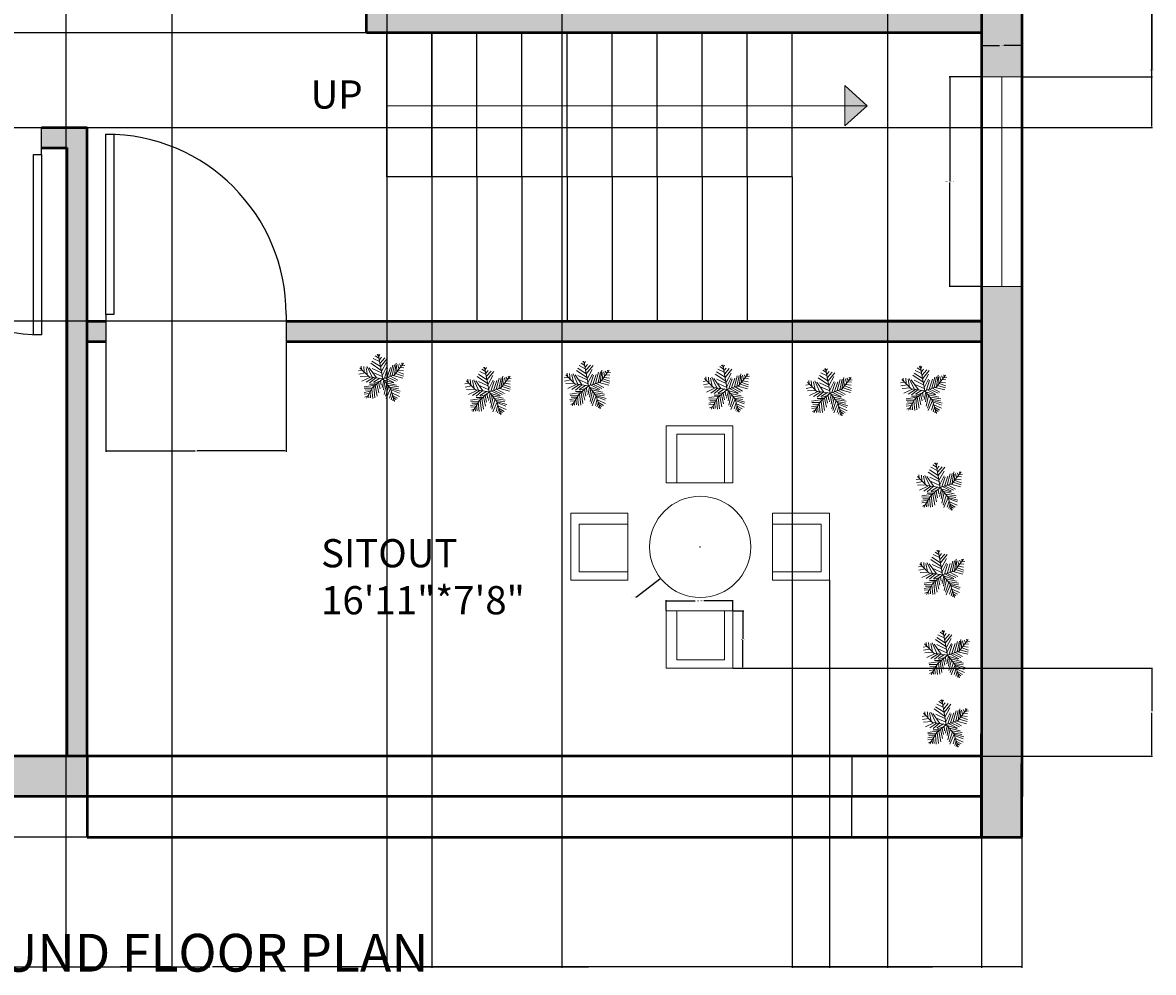
# Model space of a CAD drawing. Units: inches. Extents: x 2405 to 2823, y 1214 to 1813.
# Tile 2 of 4: x 2572 to 2823, y 1214 to 1425. Entities that reach past the tile are written whole.
import ezdxf

# ---------------------------------------------------------------- set-up
doc = ezdxf.new("R2010")
doc.units = ezdxf.units.IN
for name, color, linetype, lineweight in [('A-ANNO-DIMS', 2, 'Continuous', 18), ('A-ANNO-SYMB', 7, 'Continuous', 18), ('A-AREA-IDEN', 30, 'Continuous', 25), ('A-FLOR-STRS', 7, 'Continuous', 25), ('A-WALL-PATT', 252, 'Continuous', 13), ('DOOR', 133, 'Continuous', 25), ('FUR', 10, 'Continuous', 18), ('TEXT', 30, 'Continuous', 25), ('TREE', 90, 'Continuous', 13), ('WALL', 140, 'Continuous', 50), ('WIND', 200, 'Continuous', 18)]:
    doc.layers.add(name, color=color, linetype=linetype, lineweight=lineweight)
doc.styles.get("Standard").update_dxf_attribs({"font": 'arial.ttf'})
doc.dimstyles.get("Standard").update_dxf_attribs({"dimtxt": 0.18, "dimasz": 0.18, "dimexe": 0.18, "dimexo": 0.0625, "dimgap": 0.09, "dimtad": 0, "dimtih": 1, "dimtoh": 1, "dimdec": 4, "dimzin": 0, "dimdsep": 46, "dimtxsty": 'Standard', "dimcen": 0.09, "dimadec": 0, "dimazin": 0, "dimtfac": 1, "dimtdec": 4, "dimtofl": 0, "dimtmove": 0, "dimatfit": 3, "dimfxl": 1, "dimtolj": 1, "dimtzin": 0, "dimarcsym": 0})

# ---------------------------------------------------------------- blocks, each defined once
blk = doc.blocks.new('*U2')
for p, q in [((0, 0), (0, -6)), ((40, 0), (40, -6))]:
    blk.add_line(p, q)
blk.add_lwpolyline([(0, 0), (0, 40), (1.75, 40), (1.75, 0)], close=True)
blk.add_arc((0, 0), 40, 0, 90)
blk = doc.blocks.new('*U6')
for p, q in [((-8.737, 47.138), (-17.069, 52.711)), ((-10.186, 53.64), (-13.084, 55.962)), ((0, 0), (-10.5, 57)), ((-9.099, 51.782), (-6.563, 55.962)), ((-48.585, 21.131), (-49.309, 29.026)), ((-43.513, 28.561), (-42.427, 15.558)), ((-38.442, 26.239), (-34.819, 7.663)), ((-35.544, 28.097), (-24.314, 3.947)), ((-3.665, 19.273), (-27.574, 35.527)), ((-5.114, 28.097), (-24.676, 40.636)), ((-7.288, 39.707), (-21.778, 46.673)), ((-7.65, 43.423), (-2.578, 49.46)), ((-5.839, 35.992), (4.667, 48.067)), ((-5.114, 27.632), (10.463, 46.673)), ((-2.941, 16.486), (8.652, 37.85)), ((-1.129, 6.734), (9.014, 26.704)), ((10.101, 3.483), (17.708, 26.239)), ((16.259, 5.805), (23.142, 31.348)), ((22.055, 7.198), (27.489, 32.277)), ((27, 9), (48, 36)), ((27.127, 9.056), (31.112, 35.992)), ((31.836, 30.883), (32.561, 16.486)), ((35.096, 32.741), (37.27, 22.524)), ((38.719, 34.134), (41.979, 28.561)), ((43.791, 29.954), (51.036, 30.883)), ((44.153, 36.456), (45.239, 32.741)), ((-47.498, 19.737), (-55.83, 18.344)), ((-40.615, 13.7), (-55.105, 10.913)), ((-31.5, 4.5), (-52.5, 25.5)), ((-33.37, 6.269), (-52.207, 5.34)), ((-28.299, 3.483), (-47.86, -5.805)), ((-21.416, 3.018), (-38.079, -8.128)), ((0, 0), (-31.5, 4.5)), ((-14.533, 2.09), (-30.834, 25.31)), ((-15.982, 2.09), (-30.11, -9.521)), ((-24.314, 23.917), (-2.941, 13.7)), ((0, 0), (-22.5, -19.5)), ((-6.563, 1.161), (-21.416, -8.128)), ((-20.691, 13.7), (-1.129, 4.876)), ((0, 0), (27, 9)), ((0, 0), (18, -22.5)), ((3.942, 1.625), (11.187, 24.381)), ((6.478, 1.625), (26.04, -8.592)), ((11.187, 3.483), (30.749, -5.805)), ((18.07, 5.805), (35.096, -3.483)), ((24.229, 7.663), (46.688, 1.625)), ((29.662, 12.307), (48.137, 6.269)), ((33.285, 16.486), (48.862, 10.913)), ((36.183, 19.737), (48.137, 17.88)), ((40.53, 25.775), (48.862, 24.846)), ((-17.431, -15.094), (-42.789, -18.809)), ((-24.314, -21.596), (-42.427, -22.06)), ((-26.849, -26.24), (-40.253, -25.775)), ((-22.5, -19.5), (-37.5, -45)), ((-15.257, -12.772), (-30.11, -12.772)), ((-25.038, -23.918), (-22.865, -45.281)), ((-20.691, -18.345), (-17.793, -44.352)), ((-6.563, -5.805), (-19.967, -9.985)), ((-17.069, -15.094), (-12.721, -40.172)), ((-13.446, -11.378), (-8.737, -32.741)), ((-9.461, -8.592), (-6.201, -23.453)), ((-4.752, -3.483), (-3.665, -14.629)), ((2.493, -3.019), (-1.491, -20.202)), ((1.769, -2.555), (24.229, -9.521)), ((5.029, -6.27), (2.131, -25.775)), ((9.014, -11.378), (3.58, -35.992)), ((14.085, -16.951), (6.478, -40.172)), ((7.565, -9.056), (32.198, -14.629)), ((18.07, -22.524), (8.289, -45.745)), ((12.274, -15.094), (36.907, -18.809)), ((16.259, -19.738), (36.183, -22.989)), ((18, -22.5), (27, -52.5)), ((18.433, -22.524), (40.53, -29.026)), ((19.157, -25.311), (38.719, -33.206)), ((-28.299, -29.026), (-42.789, -31.348)), ((-30.834, -34.135), (-42.427, -35.528)), ((-34.457, -39.708), (-40.978, -42.494)), ((-32.646, -36.921), (-31.921, -44.352)), ((-29.023, -30.884), (-27.936, -43.887)), ((20.244, -30.419), (15.897, -44.816)), ((22.78, -37.85), (19.519, -48.532)), ((21.331, -32.741), (39.081, -40.636)), ((22.78, -38.314), (34.372, -44.816)), ((24.591, -45.745), (23.142, -50.854)), ((24.591, -43.423), (30.749, -47.603)), ((26.764, -49.925), (28.213, -50.854))]:
    blk.add_line(p, q)
blk = doc.blocks.new('CHAIR-SITOUT')
for p, q in [((0, 0), (0, 12.67)), ((0, 12.67), (14.84, 12.67)), ((14.84, 12.67), (14.84, 0)), ((2.41, 0), (0, 0)), ((12.99, 0), (14.84, 0))]:
    blk.add_line(p, q)
blk.add_lwpolyline([(2.41, 0), (12.99, 0), (12.99, 10.83), (2.41, 10.83)], close=True)
blk = doc.blocks.new('WIN-46_53')
blk.add_line((4.5, 0), (4.5, 46.53))
blk.add_lwpolyline([(0, 0), (9, 0), (9, 46.53), (0, 46.53)], close=True)
blk = doc.blocks.new('*D14')
at = {"layer": 'A-ANNO-DIMS', "color": 0, "lineweight": -2, "transparency": 16777216}
for p, q in [((2714.75, 1294.2), (2714.75, 1296.54)), ((2714.93, 1296.36), (2721.22, 1296.36)), ((2729.41, 1296.36), (2723.12, 1296.36)), ((2729.59, 1294.2), (2729.59, 1296.54))]:
    blk.add_line(p, q, dxfattribs=at)
at = {"layer": 'A-ANNO-DIMS', "color": 0, "lineweight": 100, "transparency": 16777216}
for points in [[(2714.93, 1296.39), (2714.93, 1296.33), (2714.75, 1296.36)], [(2729.41, 1296.39), (2729.41, 1296.33), (2729.59, 1296.36)]]:
    blk.add_solid(points, dxfattribs=at)
at = {"layer": 'Defpoints', "color": 0, "lineweight": 100, "transparency": 16777216}
for p in [(2729.59, 1296.36), (2714.75, 1294.14), (2729.59, 1294.14)]:
    blk.add_point(p, dxfattribs=at)
at = {"layer": 'A-ANNO-DIMS', "color": 0, "transparency": 16777216, "insert": (2722.17, 1296.36), "char_height": 0.18, "attachment_point": 5}
blk.add_mtext('\\A1;CHAIR 15 TYP.', dxfattribs=at)
blk = doc.blocks.new('*D15')
at = {"layer": 'A-ANNO-DIMS', "color": 0, "lineweight": -2, "transparency": 16777216}
for p, q in [((2729.65, 1294.14), (2731.99, 1294.14)), ((2731.81, 1293.96), (2731.81, 1287.98)), ((2731.81, 1281.64), (2731.81, 1287.62)), ((2729.65, 1281.46), (2731.99, 1281.46))]:
    blk.add_line(p, q, dxfattribs=at)
at = {"layer": 'A-ANNO-DIMS', "color": 0, "lineweight": 100, "transparency": 16777216}
for points in [[(2731.78, 1293.96), (2731.84, 1293.96), (2731.81, 1294.14)], [(2731.78, 1281.64), (2731.84, 1281.64), (2731.81, 1281.46)]]:
    blk.add_solid(points, dxfattribs=at)
at = {"layer": 'Defpoints', "color": 0, "lineweight": 100, "transparency": 16777216}
for p in [(2729.59, 1294.14), (2729.59, 1281.46), (2731.81, 1281.46)]:
    blk.add_point(p, dxfattribs=at)
at = {"layer": 'A-ANNO-DIMS', "color": 0, "transparency": 16777216, "insert": (2731.81, 1287.8), "char_height": 0.18, "attachment_point": 5}
blk.add_mtext('\\A1;13 TYP.', dxfattribs=at)
blk = doc.blocks.new('*D20')
at = {"layer": 'A-ANNO-DIMS', "color": 0, "lineweight": -2, "transparency": 16777216}
for p, q in [((2784.71, 1412.65), (2777.61, 1412.65)), ((2777.79, 1412.47), (2777.79, 1389.57)), ((2777.79, 1366.3), (2777.79, 1389.2)), ((2784.71, 1366.12), (2777.61, 1366.12))]:
    blk.add_line(p, q, dxfattribs=at)
at = {"layer": 'A-ANNO-DIMS', "color": 0, "lineweight": 100, "transparency": 16777216}
for points in [[(2777.76, 1412.47), (2777.82, 1412.47), (2777.79, 1412.65)], [(2777.76, 1366.3), (2777.82, 1366.3), (2777.79, 1366.12)]]:
    blk.add_solid(points, dxfattribs=at)
at = {"layer": 'Defpoints', "color": 0, "lineweight": 100, "transparency": 16777216}
for p in [(2777.79, 1412.65), (2784.77, 1412.65), (2784.77, 1366.12)]:
    blk.add_point(p, dxfattribs=at)
at = {"layer": 'A-ANNO-DIMS', "color": 0, "transparency": 16777216, "insert": (2777.79, 1389.39), "char_height": 0.18, "attachment_point": 5}
blk.add_mtext('\\A1;WINDOW 47 TYP.', dxfattribs=at)
blk = doc.blocks.new('*D21')
at = {"layer": 'A-ANNO-DIMS', "color": 0, "lineweight": -2, "transparency": 16777216}
for p, q in [((2784.77, 1412.71), (2784.77, 1419.81)), ((2784.95, 1419.63), (2788.81, 1419.63)), ((2793.59, 1419.63), (2789.73, 1419.63)), ((2793.77, 1412.71), (2793.77, 1419.81))]:
    blk.add_line(p, q, dxfattribs=at)
at = {"layer": 'A-ANNO-DIMS', "color": 0, "lineweight": 100, "transparency": 16777216}
for points in [[(2784.95, 1419.66), (2784.95, 1419.6), (2784.77, 1419.63)], [(2793.59, 1419.66), (2793.59, 1419.6), (2793.77, 1419.63)]]:
    blk.add_solid(points, dxfattribs=at)
at = {"layer": 'Defpoints', "color": 0, "lineweight": 100, "transparency": 16777216}
for p in [(2793.77, 1419.63), (2784.77, 1412.65), (2793.77, 1412.65)]:
    blk.add_point(p, dxfattribs=at)
at = {"layer": 'A-ANNO-DIMS', "color": 0, "transparency": 16777216, "insert": (2789.27, 1419.63), "char_height": 0.18, "attachment_point": 5}
blk.add_mtext('\\A1;9 TYP.', dxfattribs=at)
blk = doc.blocks.new('*D22')
at = {"layer": 'A-ANNO-DIMS', "color": 0, "lineweight": -2, "transparency": 16777216}
for p, q in [((2433.77, 1252.87), (2433.77, 1214.95)), ((2793.77, 1243.87), (2793.77, 1214.95)), ((2433.95, 1215.13), (2613.48, 1215.13)), ((2793.59, 1215.13), (2614.06, 1215.13))]:
    blk.add_line(p, q, dxfattribs=at)
at = {"layer": 'A-ANNO-DIMS', "color": 0, "lineweight": 100, "transparency": 16777216}
for points in [[(2433.95, 1215.16), (2433.95, 1215.1), (2433.77, 1215.13)], [(2793.59, 1215.16), (2793.59, 1215.1), (2793.77, 1215.13)]]:
    blk.add_solid(points, dxfattribs=at)
at = {"layer": 'Defpoints', "color": 0, "lineweight": 100, "transparency": 16777216}
for p in [(2433.77, 1252.93), (2793.77, 1243.93), (2793.77, 1215.13)]:
    blk.add_point(p, dxfattribs=at)
at = {"layer": 'A-ANNO-DIMS', "color": 0, "transparency": 16777216, "insert": (2613.77, 1215.13), "char_height": 0.18, "attachment_point": 5}
blk.add_mtext('\\A1;360', dxfattribs=at)
blk = doc.blocks.new('*D23')
at = {"layer": 'A-ANNO-DIMS', "color": 0, "lineweight": -2, "transparency": 16777216}
for p, q in [((2433.71, 1732.93), (2404.79, 1732.93)), ((2404.97, 1732.75), (2404.97, 1488.61)), ((2404.97, 1244.11), (2404.97, 1488.25)), ((2586.21, 1243.93), (2404.79, 1243.93))]:
    blk.add_line(p, q, dxfattribs=at)
at = {"layer": 'A-ANNO-DIMS', "color": 0, "lineweight": 100, "transparency": 16777216}
for points in [[(2404.94, 1732.75), (2405, 1732.75), (2404.97, 1732.93)], [(2404.94, 1244.11), (2405, 1244.11), (2404.97, 1243.93)]]:
    blk.add_solid(points, dxfattribs=at)
at = {"layer": 'Defpoints', "color": 0, "lineweight": 100, "transparency": 16777216}
for p in [(2433.77, 1732.93), (2404.97, 1243.93), (2586.27, 1243.93)]:
    blk.add_point(p, dxfattribs=at)
at = {"layer": 'A-ANNO-DIMS', "color": 0, "transparency": 16777216, "insert": (2404.97, 1488.43), "char_height": 0.18, "attachment_point": 5}
blk.add_mtext('\\A1;489', dxfattribs=at)
blk = doc.blocks.new('*D29')
at = {"layer": 'A-ANNO-DIMS', "color": 0, "lineweight": -2, "transparency": 16777216}
for p, q in [((2793.83, 1446.4), (2822.75, 1446.4)), ((2822.57, 1446.22), (2822.57, 1429.71)), ((2822.57, 1412.83), (2822.57, 1429.35)), ((2793.83, 1412.65), (2822.75, 1412.65))]:
    blk.add_line(p, q, dxfattribs=at)
at = {"layer": 'A-ANNO-DIMS', "color": 0, "lineweight": 100, "transparency": 16777216}
for points in [[(2822.54, 1446.22), (2822.6, 1446.22), (2822.57, 1446.4)], [(2822.54, 1412.83), (2822.6, 1412.83), (2822.57, 1412.65)]]:
    blk.add_solid(points, dxfattribs=at)
at = {"layer": 'Defpoints', "color": 0, "lineweight": 100, "transparency": 16777216}
for p in [(2793.77, 1446.4), (2793.77, 1412.65), (2822.57, 1412.65)]:
    blk.add_point(p, dxfattribs=at)
at = {"layer": 'A-ANNO-DIMS', "color": 0, "transparency": 16777216, "insert": (2822.57, 1429.53), "char_height": 0.18, "attachment_point": 5}
blk.add_mtext('\\A1;33.754', dxfattribs=at)
blk = doc.blocks.new('*D34')
at = {"layer": 'A-ANNO-DIMS', "color": 0, "lineweight": -2, "transparency": 16777216}
for p, q in [((2652.71, 1422.43), (2404.79, 1422.43)), ((2404.97, 1422.25), (2404.97, 1390.61)), ((2404.97, 1358.61), (2404.97, 1390.25)), ((2652.71, 1358.43), (2404.79, 1358.43))]:
    blk.add_line(p, q, dxfattribs=at)
at = {"layer": 'A-ANNO-DIMS', "color": 0, "lineweight": 100, "transparency": 16777216}
for points in [[(2404.94, 1422.25), (2405, 1422.25), (2404.97, 1422.43)], [(2404.94, 1358.61), (2405, 1358.61), (2404.97, 1358.43)]]:
    blk.add_solid(points, dxfattribs=at)
at = {"layer": 'Defpoints', "color": 0, "lineweight": 100, "transparency": 16777216}
for p in [(2404.97, 1422.43), (2652.77, 1422.43), (2652.77, 1358.43)]:
    blk.add_point(p, dxfattribs=at)
at = {"layer": 'A-ANNO-DIMS', "color": 0, "transparency": 16777216, "insert": (2404.97, 1390.43), "char_height": 0.18, "attachment_point": 5}
blk.add_mtext('\\A1;64', dxfattribs=at)
blk = doc.blocks.new('*D35')
at = {"layer": 'A-ANNO-DIMS', "color": 0, "lineweight": -2, "transparency": 16777216}
for p, q in [((2652.77, 1358.37), (2652.77, 1214.95)), ((2742.77, 1358.37), (2742.77, 1214.95)), ((2652.95, 1215.13), (2697.55, 1215.13)), ((2742.59, 1215.13), (2697.99, 1215.13))]:
    blk.add_line(p, q, dxfattribs=at)
at = {"layer": 'A-ANNO-DIMS', "color": 0, "lineweight": 100, "transparency": 16777216}
for points in [[(2652.95, 1215.16), (2652.95, 1215.1), (2652.77, 1215.13)], [(2742.59, 1215.16), (2742.59, 1215.1), (2742.77, 1215.13)]]:
    blk.add_solid(points, dxfattribs=at)
at = {"layer": 'Defpoints', "color": 0, "lineweight": 100, "transparency": 16777216}
for p in [(2652.77, 1358.43), (2742.77, 1358.43), (2742.77, 1215.13)]:
    blk.add_point(p, dxfattribs=at)
at = {"layer": 'A-ANNO-DIMS', "color": 0, "transparency": 16777216, "insert": (2697.77, 1215.13), "char_height": 0.18, "attachment_point": 5}
blk.add_mtext('\\A1;90', dxfattribs=at)
blk = doc.blocks.new('*D36')
at = {"layer": 'A-ANNO-DIMS', "color": 0, "lineweight": -2, "transparency": 16777216}
for p, q in [((2742.77, 1358.37), (2742.77, 1214.95)), ((2784.77, 1358.37), (2784.77, 1214.95)), ((2742.95, 1215.13), (2763.55, 1215.13)), ((2784.59, 1215.13), (2763.99, 1215.13))]:
    blk.add_line(p, q, dxfattribs=at)
at = {"layer": 'A-ANNO-DIMS', "color": 0, "lineweight": 100, "transparency": 16777216}
for points in [[(2742.95, 1215.16), (2742.95, 1215.1), (2742.77, 1215.13)], [(2784.59, 1215.16), (2784.59, 1215.1), (2784.77, 1215.13)]]:
    blk.add_solid(points, dxfattribs=at)
at = {"layer": 'Defpoints', "color": 0, "lineweight": 100, "transparency": 16777216}
for p in [(2742.77, 1358.43), (2784.77, 1358.43), (2784.77, 1215.13)]:
    blk.add_point(p, dxfattribs=at)
at = {"layer": 'A-ANNO-DIMS', "color": 0, "transparency": 16777216, "insert": (2763.77, 1215.13), "char_height": 0.18, "attachment_point": 5}
blk.add_mtext('\\A1;42', dxfattribs=at)
blk = doc.blocks.new('*D37')
at = {"layer": 'A-ANNO-DIMS', "color": 0, "lineweight": -2, "transparency": 16777216}
for p, q in [((2652.77, 1422.37), (2652.77, 1214.95)), ((2662.77, 1422.37), (2662.77, 1214.95)), ((2652.95, 1215.13), (2657.56, 1215.13)), ((2662.59, 1215.13), (2657.98, 1215.13))]:
    blk.add_line(p, q, dxfattribs=at)
at = {"layer": 'A-ANNO-DIMS', "color": 0, "lineweight": 100, "transparency": 16777216}
for points in [[(2652.95, 1215.16), (2652.95, 1215.1), (2652.77, 1215.13)], [(2662.59, 1215.16), (2662.59, 1215.1), (2662.77, 1215.13)]]:
    blk.add_solid(points, dxfattribs=at)
at = {"layer": 'Defpoints', "color": 0, "lineweight": 100, "transparency": 16777216}
for p in [(2652.77, 1422.43), (2662.77, 1422.43), (2662.77, 1215.13)]:
    blk.add_point(p, dxfattribs=at)
at = {"layer": 'A-ANNO-DIMS', "color": 0, "transparency": 16777216, "insert": (2657.77, 1215.13), "char_height": 0.18, "attachment_point": 5}
blk.add_mtext('\\A1;10', dxfattribs=at)
blk = doc.blocks.new('*D40')
at = {"layer": 'A-ANNO-DIMS', "color": 0, "lineweight": -2, "transparency": 16777216}
for p, q in [((2652.77, 1426.87), (2652.77, 1214.95)), ((2691.63, 1426.87), (2691.63, 1214.95)), ((2652.95, 1215.13), (2671.8, 1215.13)), ((2691.45, 1215.13), (2672.59, 1215.13))]:
    blk.add_line(p, q, dxfattribs=at)
at = {"layer": 'A-ANNO-DIMS', "color": 0, "lineweight": 100, "transparency": 16777216}
for points in [[(2652.95, 1215.16), (2652.95, 1215.1), (2652.77, 1215.13)], [(2691.45, 1215.16), (2691.45, 1215.1), (2691.63, 1215.13)]]:
    blk.add_solid(points, dxfattribs=at)
at = {"layer": 'Defpoints', "color": 0, "lineweight": 100, "transparency": 16777216}
for p in [(2652.77, 1426.93), (2691.63, 1426.93), (2691.63, 1215.13)]:
    blk.add_point(p, dxfattribs=at)
at = {"layer": 'A-ANNO-DIMS', "color": 0, "transparency": 16777216, "insert": (2672.2, 1215.13), "char_height": 0.18, "attachment_point": 5}
blk.add_mtext('\\A1;38.86', dxfattribs=at)
blk = doc.blocks.new('*D42')
at = {"layer": 'A-ANNO-DIMS', "color": 0, "lineweight": -2, "transparency": 16777216}
for p, q in [((2581.53, 1614.9), (2581.53, 1214.95)), ((2605.03, 1615.87), (2605.03, 1214.95)), ((2581.71, 1215.13), (2592.95, 1215.13)), ((2604.85, 1215.13), (2593.61, 1215.13))]:
    blk.add_line(p, q, dxfattribs=at)
at = {"layer": 'A-ANNO-DIMS', "color": 0, "lineweight": 100, "transparency": 16777216}
for points in [[(2581.71, 1215.16), (2581.71, 1215.1), (2581.53, 1215.13)], [(2604.85, 1215.16), (2604.85, 1215.1), (2605.03, 1215.13)]]:
    blk.add_solid(points, dxfattribs=at)
at = {"layer": 'Defpoints', "color": 0, "lineweight": 100, "transparency": 16777216}
for p in [(2581.53, 1614.96), (2605.03, 1615.93), (2605.03, 1215.13)]:
    blk.add_point(p, dxfattribs=at)
at = {"layer": 'A-ANNO-DIMS', "color": 0, "transparency": 16777216, "insert": (2593.28, 1215.13), "char_height": 0.18, "attachment_point": 5}
blk.add_mtext('\\A1;23.5', dxfattribs=at)
blk = doc.blocks.new('*D43')
at = {"layer": 'A-ANNO-DIMS', "color": 0, "lineweight": -2, "transparency": 16777216}
for p, q in [((2590.41, 1358.37), (2590.41, 1329.45)), ((2630.41, 1358.37), (2630.41, 1329.45)), ((2590.59, 1329.63), (2610.18, 1329.63)), ((2630.23, 1329.63), (2610.63, 1329.63))]:
    blk.add_line(p, q, dxfattribs=at)
at = {"layer": 'A-ANNO-DIMS', "color": 0, "lineweight": 100, "transparency": 16777216}
for points in [[(2590.59, 1329.66), (2590.59, 1329.6), (2590.41, 1329.63)], [(2630.23, 1329.66), (2630.23, 1329.6), (2630.41, 1329.63)]]:
    blk.add_solid(points, dxfattribs=at)
at = {"layer": 'Defpoints', "color": 0, "lineweight": 100, "transparency": 16777216}
for p in [(2590.41, 1358.43), (2630.41, 1358.43), (2590.41, 1329.63)]:
    blk.add_point(p, dxfattribs=at)
at = {"layer": 'A-ANNO-DIMS', "color": 0, "transparency": 16777216, "insert": (2610.41, 1329.63), "char_height": 0.18, "attachment_point": 5}
blk.add_mtext('\\A1;40', dxfattribs=at)
blk = doc.blocks.new('*D48')
at = {"layer": 'A-ANNO-DIMS', "color": 0, "lineweight": -2, "transparency": 16777216}
for p, q in [((2763.95, 1463.41), (2763.95, 1214.95)), ((2784.77, 1463.41), (2784.77, 1214.95)), ((2764.13, 1215.13), (2773.9, 1215.13)), ((2784.59, 1215.13), (2774.83, 1215.13))]:
    blk.add_line(p, q, dxfattribs=at)
at = {"layer": 'A-ANNO-DIMS', "color": 0, "lineweight": 100, "transparency": 16777216}
for points in [[(2764.13, 1215.16), (2764.13, 1215.1), (2763.95, 1215.13)], [(2784.59, 1215.16), (2784.59, 1215.1), (2784.77, 1215.13)]]:
    blk.add_solid(points, dxfattribs=at)
at = {"layer": 'Defpoints', "color": 0, "lineweight": 100, "transparency": 16777216}
for p in [(2763.95, 1463.47), (2784.77, 1463.47), (2784.77, 1215.13)]:
    blk.add_point(p, dxfattribs=at)
at = {"layer": 'A-ANNO-DIMS', "color": 0, "transparency": 16777216, "insert": (2774.36, 1215.13), "char_height": 0.18, "attachment_point": 5}
blk.add_mtext('\\A1;20.813', dxfattribs=at)
blk = doc.blocks.new('*D50')
at = {"layer": 'A-ANNO-DIMS', "color": 0, "lineweight": -2, "transparency": 16777216}
for p, q in [((2477.36, 1427.01), (2822.75, 1427.01)), ((2822.57, 1426.83), (2822.57, 1414.4)), ((2822.57, 1401.61), (2822.57, 1414.04)), ((2442.83, 1401.43), (2822.75, 1401.43))]:
    blk.add_line(p, q, dxfattribs=at)
at = {"layer": 'A-ANNO-DIMS', "color": 0, "lineweight": 100, "transparency": 16777216}
for points in [[(2822.54, 1426.83), (2822.6, 1426.83), (2822.57, 1427.01)], [(2822.54, 1401.61), (2822.6, 1401.61), (2822.57, 1401.43)]]:
    blk.add_solid(points, dxfattribs=at)
at = {"layer": 'Defpoints', "color": 0, "lineweight": 100, "transparency": 16777216}
for p in [(2477.3, 1427.01), (2822.57, 1427.01), (2442.77, 1401.43)]:
    blk.add_point(p, dxfattribs=at)
at = {"layer": 'A-ANNO-DIMS', "color": 0, "transparency": 16777216, "insert": (2822.57, 1414.22), "char_height": 0.18, "attachment_point": 5}
blk.add_mtext('\\A1;25.584', dxfattribs=at)
blk = doc.blocks.new('*D60')
at = {"layer": 'A-ANNO-DIMS', "color": 0, "lineweight": -2, "transparency": 16777216}
for p, q in [((2751.03, 1300.93), (2751.03, 1214.95)), ((2784.77, 1261.87), (2784.77, 1214.95)), ((2751.21, 1215.13), (2767.5, 1215.13)), ((2784.59, 1215.13), (2768.29, 1215.13))]:
    blk.add_line(p, q, dxfattribs=at)
at = {"layer": 'A-ANNO-DIMS', "color": 0, "lineweight": 100, "transparency": 16777216}
for points in [[(2751.21, 1215.16), (2751.21, 1215.1), (2751.03, 1215.13)], [(2784.59, 1215.16), (2784.59, 1215.1), (2784.77, 1215.13)]]:
    blk.add_solid(points, dxfattribs=at)
at = {"layer": 'Defpoints', "color": 0, "lineweight": 100, "transparency": 16777216}
for p in [(2751.03, 1300.99), (2784.77, 1261.93), (2751.03, 1215.13)]:
    blk.add_point(p, dxfattribs=at)
at = {"layer": 'A-ANNO-DIMS', "color": 0, "transparency": 16777216, "insert": (2767.9, 1215.13), "char_height": 0.18, "attachment_point": 5}
blk.add_mtext('\\A1;33.74', dxfattribs=at)
blk = doc.blocks.new('*D61')
at = {"layer": 'A-ANNO-DIMS', "color": 0, "lineweight": -2, "transparency": 16777216}
for p, q in [((2729.65, 1281.46), (2822.75, 1281.46)), ((2822.57, 1281.28), (2822.57, 1271.88)), ((2822.57, 1262.11), (2822.57, 1271.51)), ((2784.83, 1261.93), (2822.75, 1261.93))]:
    blk.add_line(p, q, dxfattribs=at)
at = {"layer": 'A-ANNO-DIMS', "color": 0, "lineweight": 100, "transparency": 16777216}
for points in [[(2822.54, 1281.28), (2822.6, 1281.28), (2822.57, 1281.46)], [(2822.54, 1262.11), (2822.6, 1262.11), (2822.57, 1261.93)]]:
    blk.add_solid(points, dxfattribs=at)
at = {"layer": 'Defpoints', "color": 0, "lineweight": 100, "transparency": 16777216}
for p in [(2729.59, 1281.46), (2822.57, 1281.46), (2784.77, 1261.93)]:
    blk.add_point(p, dxfattribs=at)
at = {"layer": 'A-ANNO-DIMS', "color": 0, "transparency": 16777216, "insert": (2822.57, 1271.7), "char_height": 0.18, "attachment_point": 5}
blk.add_mtext('\\A1;19.533', dxfattribs=at)
blk = doc.blocks.new('*D69')
at = {"layer": 'A-ANNO-DIMS', "color": 0, "lineweight": -2, "transparency": 16777216}
for p, q in [((2784.71, 1261.93), (2755.79, 1261.93)), ((2755.97, 1261.75), (2755.97, 1253.11)), ((2755.97, 1244.11), (2755.97, 1252.75)), ((2784.71, 1243.93), (2755.79, 1243.93))]:
    blk.add_line(p, q, dxfattribs=at)
at = {"layer": 'A-ANNO-DIMS', "color": 0, "lineweight": 100, "transparency": 16777216}
for points in [[(2755.94, 1261.75), (2756, 1261.75), (2755.97, 1261.93)], [(2755.94, 1244.11), (2756, 1244.11), (2755.97, 1243.93)]]:
    blk.add_solid(points, dxfattribs=at)
at = {"layer": 'Defpoints', "color": 0, "lineweight": 100, "transparency": 16777216}
for p in [(2755.97, 1261.93), (2784.77, 1261.93), (2784.77, 1243.93)]:
    blk.add_point(p, dxfattribs=at)
at = {"layer": 'A-ANNO-DIMS', "color": 0, "transparency": 16777216, "insert": (2755.97, 1252.93), "char_height": 0.18, "attachment_point": 5}
blk.add_mtext('\\A1;18', dxfattribs=at)
blk = doc.blocks.new('*D70')
at = {"layer": 'A-ANNO-DIMS', "color": 0, "lineweight": -2, "transparency": 16777216}
for p, q in [((2722.24, 1308.35), (2722.42, 1308.35)), ((2722.33, 1308.26), (2722.33, 1308.44)), ((2708.22, 1297.24), (2713.37, 1301.29)), ((2708.04, 1297.24), (2708.22, 1297.24))]:
    blk.add_line(p, q, dxfattribs=at)
at = {"layer": 'A-ANNO-DIMS', "color": 0, "lineweight": 100, "transparency": 16777216}
blk.add_solid([(2713.35, 1301.32), (2713.39, 1301.27), (2713.51, 1301.4)], dxfattribs=at)
at = {"layer": 'Defpoints', "color": 0, "lineweight": 100, "transparency": 16777216}
for p in [(2731.15, 1315.29), (2713.51, 1301.4)]:
    blk.add_point(p, dxfattribs=at)
at = {"layer": 'A-ANNO-DIMS', "color": 0, "transparency": 16777216, "insert": (2707.48, 1297.24), "char_height": 0.18, "attachment_point": 5}
blk.add_mtext('\\A1;∅22.447', dxfattribs=at)

msp = doc.modelspace()

# ---------------------------------------------------------------- hatches: boundary and pattern name
at = {"layer": 'A-ANNO-SYMB'}
h = msp.add_hatch(color=256, dxfattribs=at)
h.dxf.hatch_style = 1
h.paths.add_polyline_path([(2754.4666, 1410.736), (2754.4666, 1406.252), (2759.4319, 1406.252)])
h.paths.add_polyline_path([(2759.4319, 1406.252), (2754.4666, 1406.252), (2754.4666, 1401.7681)])
at = {"layer": 'A-WALL-PATT'}
h = msp.add_hatch(color=256, dxfattribs=at)
h.dxf.hatch_style = 1
h.paths.add_polyline_path([(2601.7679, 1732.9303), (2433.7679, 1732.9303), (2433.7679, 1680.7368), (2442.7679, 1680.7368), (2442.7679, 1723.9303), (2574.7679, 1723.9303), (2601.7679, 1723.9303)])
h.paths.add_polyline_path([(2793.7679, 1732.9303), (2622.7552, 1732.9303), (2622.7552, 1723.9303), (2622.7679, 1723.9303), (2645.2679, 1723.9303), (2784.7679, 1723.9303), (2784.7679, 1680.7368), (2793.7679, 1680.7368)])
h.paths.add_polyline_path([(2442.7679, 1605.111), (2433.7679, 1605.111), (2433.7679, 1513.1454), (2442.7679, 1513.1454), (2442.7679, 1563.4303)])
h.paths.add_polyline_path([(2531.8067, 1567.9303), (2442.7679, 1567.9303), (2442.7679, 1563.4303), (2531.8067, 1563.4303)])
h.paths.add_polyline_path([(2793.7679, 1605.111), (2784.7679, 1605.111), (2784.7679, 1555.6662), (2793.7679, 1555.6662)])
h.paths.add_polyline_path([(2784.7679, 1567.9303), (2691.5187, 1567.9303), (2691.5187, 1563.4303), (2784.7679, 1563.4303)])
h.paths.add_polyline_path([(2649.7679, 1611.4303), (2645.2679, 1611.4303), (2645.2679, 1563.4303), (2651.5187, 1563.4303), (2651.5187, 1567.9303), (2649.7679, 1567.9303)])
h.paths.add_polyline_path([(2581.5294, 1614.9584), (2581.5294, 1615.9303), (2579.2679, 1615.9303), (2579.2679, 1611.4303), (2581.5294, 1611.4303)])
h.paths.add_polyline_path([(2579.2679, 1723.9303), (2574.7679, 1723.9303), (2574.7679, 1567.9303), (2571.8067, 1567.9303), (2571.8067, 1563.4303), (2579.2679, 1563.4303)])
h.paths.add_polyline_path([(2649.7679, 1723.9303), (2645.2679, 1723.9303), (2645.2679, 1615.9303), (2605.0298, 1615.9303, -0.01033406), (2605.0499, 1614.9584), (2605.0499, 1611.4303), (2649.7679, 1611.4303)])
h.paths.add_polyline_path([(2793.7679, 1523.737), (2784.7679, 1523.737), (2784.7679, 1492.9303), (2793.7679, 1492.9303)])
h.paths.add_polyline_path([(2793.7679, 1446.4039), (2784.7679, 1446.4039), (2784.7679, 1426.9303), (2784.7679, 1412.6503), (2793.7679, 1412.6503)])
h.paths.add_polyline_path([(2652.7679, 1467.3906), (2648.2679, 1467.3906), (2648.2679, 1422.4303), (2784.7679, 1422.4303), (2784.7679, 1426.9303), (2652.7679, 1426.9303)])
h.paths.add_polyline_path([(2696.2679, 1515.4303), (2648.2679, 1515.4303), (2648.2679, 1507.3906), (2652.7679, 1507.3906), (2652.7679, 1510.9303), (2696.2679, 1510.9303)])
h.paths.add_polyline_path([(2784.7679, 1515.4303), (2700.7679, 1515.4303), (2696.2679, 1515.4303), (2696.2679, 1510.9303), (2784.7679, 1510.9303)])
h.paths.add_polyline_path([(2700.7679, 1522.7934), (2696.2679, 1522.7934), (2696.2679, 1515.4303), (2700.7679, 1515.4303)])
h.paths.add_polyline_path([(2700.7679, 1563.4303), (2696.2679, 1563.4303), (2696.2679, 1557.1044), (2700.7679, 1557.1044)])
h.paths.add_polyline_path([(2442.7679, 1437.5196), (2433.7679, 1437.5196), (2433.7679, 1252.9303), (2481.6786, 1252.9303), (2481.6786, 1261.9303), (2442.7679, 1261.9303)])
h.paths.add_polyline_path([(2536.0913, 1401.4303), (2442.7679, 1401.4303), (2442.7679, 1396.9303), (2536.0913, 1396.9303)])
h.paths.add_polyline_path([(2784.7679, 1358.4303), (2630.4061, 1358.4303), (2630.4061, 1353.9303), (2784.7679, 1353.9303)])
h.paths.add_polyline_path([(2793.7679, 1366.1239), (2784.7679, 1366.1239), (2784.7679, 1261.9303), (2784.7679, 1243.9303), (2793.7679, 1243.9303), (2793.7679, 1260.2097)])
h.paths.add_polyline_path([(2590.4061, 1358.4303), (2586.2679, 1358.4303), (2586.2679, 1353.9303), (2590.4061, 1353.9303)])
h.paths.add_polyline_path([(2586.2679, 1353.9303), (2586.2679, 1401.4303), (2576.0913, 1401.4303), (2576.0913, 1396.9303), (2581.7679, 1396.9303), (2581.7679, 1261.9303), (2586.2679, 1261.9303)])
h.paths.add_polyline_path([(2586.2679, 1261.9303), (2581.7679, 1261.9303), (2550.8023, 1261.9303), (2550.8023, 1252.9303), (2586.2679, 1252.9303)])

# ---------------------------------------------------------------- linework, layer by layer
at = {"layer": 'A-ANNO-SYMB'}
for p, q in [((2759.4319, 1406.252), (2754.4666, 1410.736)), ((2754.4666, 1401.7681), (2754.4666, 1410.736)), ((2652.7679, 1406.252), (2759.4319, 1406.252)), ((2759.4319, 1406.252), (2754.4666, 1401.7681))]:
    msp.add_line(p, q, dxfattribs=at)
at = {"layer": 'A-FLOR-STRS'}
for p, q in [((2652.7679, 1390.4303), (2652.7679, 1422.4303)), ((2662.7679, 1390.4303), (2662.7679, 1422.4303)), ((2672.7679, 1390.4303), (2672.7679, 1422.4303)), ((2682.7679, 1390.4303), (2682.7679, 1422.4303)), ((2692.7679, 1390.4303), (2692.7679, 1422.4303)), ((2702.7679, 1390.4303), (2702.7679, 1422.4303)), ((2712.7679, 1390.4303), (2712.7679, 1422.4303)), ((2722.7679, 1390.4303), (2722.7679, 1422.4303)), ((2732.7679, 1390.4303), (2732.7679, 1422.4303)), ((2742.7679, 1390.4303), (2742.7679, 1422.4303)), ((2742.7679, 1390.4303), (2652.7679, 1390.4303)), ((2652.7679, 1390.4303), (2652.7679, 1358.4303)), ((2662.7679, 1390.4303), (2662.7679, 1358.4303)), ((2672.7679, 1390.4303), (2672.7679, 1358.4303)), ((2682.7679, 1390.4303), (2682.7679, 1358.4303)), ((2692.7679, 1390.4303), (2692.7679, 1358.4303)), ((2702.7679, 1390.4303), (2702.7679, 1358.4303)), ((2712.7679, 1390.4303), (2712.7679, 1358.4303)), ((2722.7679, 1390.4303), (2722.7679, 1358.4303)), ((2732.7679, 1390.4303), (2732.7679, 1358.4303)), ((2742.7679, 1390.4303), (2742.7679, 1358.4303))]:
    msp.add_line(p, q, dxfattribs=at)
at = {"layer": 'FUR'}
msp.add_circle((2722.3305, 1308.3471), 11.2234, dxfattribs=at)
at = {"layer": 'WALL'}
for p, q in [((2793.7679, 1732.9303), (2793.7679, 1252.9303)), ((2784.7679, 1723.9303), (2784.7679, 1261.9303)), ((2648.2679, 1422.4303), (2648.2679, 1467.3906)), ((2784.7679, 1422.4303), (2648.2679, 1422.4303)), ((2576.0913, 1401.4303), (2586.2679, 1401.4303)), ((2586.2679, 1261.9303), (2586.2679, 1401.4303)), ((2576.0913, 1396.9303), (2581.7679, 1396.9303)), ((2581.7679, 1261.9303), (2581.7679, 1396.9303)), ((2586.2679, 1358.4303), (2590.4061, 1358.4303)), ((2630.4061, 1358.4303), (2784.7679, 1358.4303)), ((2784.7679, 1358.4303), (2742.7679, 1358.4303)), ((2586.2679, 1261.9303), (2586.2679, 1353.9303)), ((2586.2679, 1353.9303), (2590.4061, 1353.9303)), ((2630.4061, 1353.9303), (2784.7679, 1353.9303)), ((2784.7679, 1243.9303), (2784.7679, 1266.8512)), ((2784.7679, 1266.8512), (2784.7679, 1243.9303)), ((2784.7679, 1261.9303), (2442.7679, 1261.9303)), ((2784.7679, 1261.9303), (2581.7679, 1261.9303)), ((2586.2679, 1261.9303), (2586.2679, 1252.9303)), ((2793.7679, 1243.9303), (2793.7679, 1260.2097)), ((2784.7679, 1252.9303), (2433.7679, 1252.9303)), ((2586.2679, 1252.9303), (2586.2679, 1243.9303)), ((2586.2679, 1243.9303), (2784.7679, 1243.9303)), ((2784.7679, 1243.9303), (2793.7679, 1243.9303))]:
    msp.add_line(p, q, dxfattribs=at)

# ---------------------------------------------------------------- block references
at = {"layer": 'DOOR', "rotation": 180}
msp.add_blockref('*U2', (2576.0913, 1395.4303), dxfattribs=at)
at = {"layer": 'DOOR'}
msp.add_blockref('*U2', (2590.4061, 1359.9303), dxfattribs=at)
at = {"layer": 'FUR'}
msp.add_blockref('CHAIR-SITOUT', (2714.749, 1322.559), dxfattribs=at)
at = {"layer": 'FUR', "extrusion": (0, 0, -1), "zscale": -1}
for p, rotation in [((-2706.3048, 1315.8336), 269.9999999999983), ((-2714.749, 1294.1351), 180)]:
    msp.add_blockref('CHAIR-SITOUT', p, dxfattribs=dict(at, rotation=rotation))
at = {"layer": 'FUR', "rotation": 270.0000000000033}
msp.add_blockref('CHAIR-SITOUT', (2738.3562, 1315.8336), dxfattribs=at)
at = {"layer": 'TREE', "xscale": 0.096295106106515, "yscale": 0.096295106106515, "zscale": 0.096295106106515}
for p in [(2651.8468, 1345.6592), (2675.4875, 1342.7399), (2697.5343, 1344.0669), (2728.3469, 1343.2707), (2772.175, 1343.0053), (2751.1906, 1342.4745), (2775.6282, 1321.5085), (2776.1594, 1302.1348), (2777.2219, 1284.3535), (2776.9563, 1268.9607)]:
    msp.add_blockref('*U6', p, dxfattribs=at)
at = {"layer": 'WIND'}
msp.add_blockref('WIN-46_53', (2784.768, 1366.124), dxfattribs=at)

# ---------------------------------------------------------------- texts
at = {"layer": 'A-AREA-IDEN', "insert": (2638.1638, 1310.0666), "char_height": 6.256044, "attachment_point": 1}
msp.add_mtext_dynamic_manual_height_columns('SITOUT\\P16\'11"*7\'8"', width=135.493128, gutter_width=31.2802, heights=[0], dxfattribs=at)
at = {"layer": 'TEXT', "attachment_point": 1}
for s, width, gutter_width, insert, char_height in [('UP', 135.493128, 31.2802, (2635.8321, 1411.8607), 6.25604), ('GROUND FLOOR PLAN', 725.174894, 41.9899, (2543.2701, 1222.4779), 8.397982)]:
    msp.add_mtext_dynamic_manual_height_columns(s, width=width, gutter_width=gutter_width, heights=[0], dxfattribs=dict(at, insert=insert, char_height=char_height))

# ---------------------------------------------------------------- dimensions: what is measured, and where the dimension line sits
at = {"layer": 'A-ANNO-DIMS'}
for base, p1, p2, angle, override, picture, middle in [((2404.9679, 1243.9303), (2433.7679, 1732.9303), (2586.2679, 1243.9303), 90, {"dimdec": 0, "dimlfac": 1, "dimrnd": 0, "dimzin": 0, "dimdsep": 46, "dimlunit": 2}, '*D23', (2404.9679, 1488.4303)), ((2822.5679, 1412.6503), (2793.7679, 1446.4039), (2793.7679, 1412.6503), 90, {"dimdec": 3, "dimlfac": 1, "dimrnd": 0, "dimzin": 0, "dimdsep": 46, "dimlunit": 2}, '*D29', (2822.5679, 1429.5271)), ((2822.5679, 1427.0139), (2442.7679, 1401.4303), (2477.2955, 1427.0139), 90, {"dimdec": 3, "dimlfac": 1, "dimrnd": 0, "dimzin": 0, "dimdsep": 46, "dimlunit": 2}, '*D50', (2822.5679, 1414.2221)), ((2404.9679, 1422.4303), (2652.7679, 1358.4303), (2652.7679, 1422.4303), 90, {"dimdec": 0, "dimlfac": 1, "dimrnd": 0, "dimzin": 0, "dimdsep": 46, "dimlunit": 2}, '*D34', (2404.9679, 1390.4303)), ((2590.4061, 1329.6303), (2630.4061, 1358.4303), (2590.4061, 1358.4303), 180, {"dimdec": 0, "dimlfac": 1, "dimrnd": 0, "dimzin": 0, "dimdsep": 46, "dimlunit": 2}, '*D43', (2610.4061, 1329.6303)), ((2822.5679, 1281.4635), (2784.7679, 1261.9303), (2729.5889, 1281.4635), 90, {"dimdec": 3, "dimlfac": 1, "dimrnd": 0, "dimzin": 0, "dimdsep": 46, "dimlunit": 2}, '*D61', (2822.5679, 1271.6969)), ((2755.9679, 1261.9303), (2784.7679, 1243.9303), (2784.7679, 1261.9303), 90, {"dimdec": 0, "dimlfac": 1, "dimrnd": 0, "dimzin": 0, "dimdsep": 46, "dimlunit": 2}, '*D69', (2755.9679, 1252.9303))]:
    dim = msp.add_linear_dim(base=base, p1=p1, p2=p2, angle=angle, dimstyle='Standard', override=override, dxfattribs=at)
    dim.commit()
    dim.dimension.update_dxf_attribs({"geometry": picture, "text_midpoint": middle})
for base, p1, p2, override, picture, middle in [((2605.0298, 1215.1303), (2581.5294, 1614.9584), (2605.0298, 1615.9303), {"dimdec": 1, "dimlfac": 1, "dimrnd": 0, "dimzin": 0, "dimdsep": 46, "dimlunit": 2}, '*D42', (2593.2796, 1215.1303)), ((2784.7679, 1215.1303), (2763.9547, 1463.4703), (2784.7679, 1463.4703), {"dimdec": 3, "dimlfac": 1, "dimrnd": 0, "dimzin": 0, "dimdsep": 46, "dimlunit": 2}, '*D48', (2774.3613, 1215.1303)), ((2691.6289, 1215.1303), (2652.7679, 1426.9303), (2691.6289, 1426.9303), {"dimdec": 2, "dimlfac": 1, "dimrnd": 0, "dimzin": 0, "dimdsep": 46, "dimlunit": 2}, '*D40', (2672.1984, 1215.1303)), ((2662.7679, 1215.1303), (2652.7679, 1422.4303), (2662.7679, 1422.4303), {"dimdec": 0, "dimlfac": 1, "dimrnd": 0, "dimzin": 0, "dimdsep": 46, "dimlunit": 2}, '*D37', (2657.7679, 1215.1303)), ((2742.7679, 1215.1303), (2652.7679, 1358.4303), (2742.7679, 1358.4303), {"dimdec": 0, "dimlfac": 1, "dimrnd": 0, "dimzin": 0, "dimdsep": 46, "dimlunit": 2}, '*D35', (2697.7679, 1215.1303)), ((2784.7679, 1215.1303), (2742.7679, 1358.4303), (2784.7679, 1358.4303), {"dimdec": 0, "dimlfac": 1, "dimrnd": 0, "dimzin": 0, "dimdsep": 46, "dimlunit": 2}, '*D36', (2763.7679, 1215.1303)), ((2751.0278, 1215.1303), (2784.7679, 1261.9303), (2751.0278, 1300.9937), {"dimdec": 2, "dimlfac": 1, "dimrnd": 0, "dimzin": 0, "dimdsep": 46, "dimlunit": 2}, '*D60', (2767.8979, 1215.1303)), ((2793.7679, 1215.1303), (2433.7679, 1252.9303), (2793.7679, 1243.9303), {"dimdec": 0, "dimlfac": 1, "dimrnd": 0, "dimzin": 0, "dimdsep": 46, "dimlunit": 2}, '*D22', (2613.7679, 1215.1303))]:
    dim = msp.add_linear_dim(base=base, p1=p1, p2=p2, dimstyle='Standard', override=override, dxfattribs=at)
    dim.commit()
    dim.dimension.update_dxf_attribs({"geometry": picture, "text_midpoint": middle})
for base, p1, p2, text, picture, middle in [((2793.7679, 1419.6292), (2784.7679, 1412.6503), (2793.7679, 1412.6503), '<> TYP.', '*D21', (2789.2679, 1419.6292)), ((2729.5889, 1296.3611), (2714.749, 1294.1351), (2729.5889, 1294.1351), 'CHAIR <> TYP.', '*D14', (2722.169, 1296.3611))]:
    dim = msp.add_linear_dim(base=base, p1=p1, p2=p2, text=text, dimstyle='Standard', override={"dimdec": 0, "dimlfac": 1, "dimrnd": 0, "dimzin": 0, "dimdsep": 46, "dimlunit": 2}, dxfattribs=at)
    dim.commit()
    dim.dimension.update_dxf_attribs({"geometry": picture, "text_midpoint": middle})
for base, p1, p2, angle, text, picture, middle in [((2777.789, 1412.6503), (2784.7679, 1366.1239), (2784.7679, 1412.6503), 90, 'WINDOW <> TYP.', '*D20', (2777.789, 1389.3871)), ((2731.8149, 1281.4635), (2729.5889, 1294.1351), (2729.5889, 1281.4635), 270, '<> TYP.', '*D15', (2731.8149, 1287.7993))]:
    dim = msp.add_linear_dim(base=base, p1=p1, p2=p2, angle=angle, text=text, dimstyle='Standard', override={"dimdec": 0, "dimlfac": 1, "dimrnd": 0, "dimzin": 0, "dimdsep": 46, "dimlunit": 2}, dxfattribs=at)
    dim.commit()
    dim.dimension.update_dxf_attribs({"geometry": picture, "text_midpoint": middle})
dim = msp.add_diameter_dim_2p(p1=(2731.1483, 1315.2905), p2=(2713.5126, 1301.4037), dimstyle='Standard', override={"dimdec": 3, "dimlfac": 1, "dimrnd": 0, "dimzin": 0, "dimdsep": 46, "dimlunit": 2}, dxfattribs=at)
dim.commit()
dim.dimension.update_dxf_attribs({"geometry": '*D70', "text_midpoint": (2707.4804, 1297.2376), "dimtype": 163})

doc.saveas('drawing.dxf')
